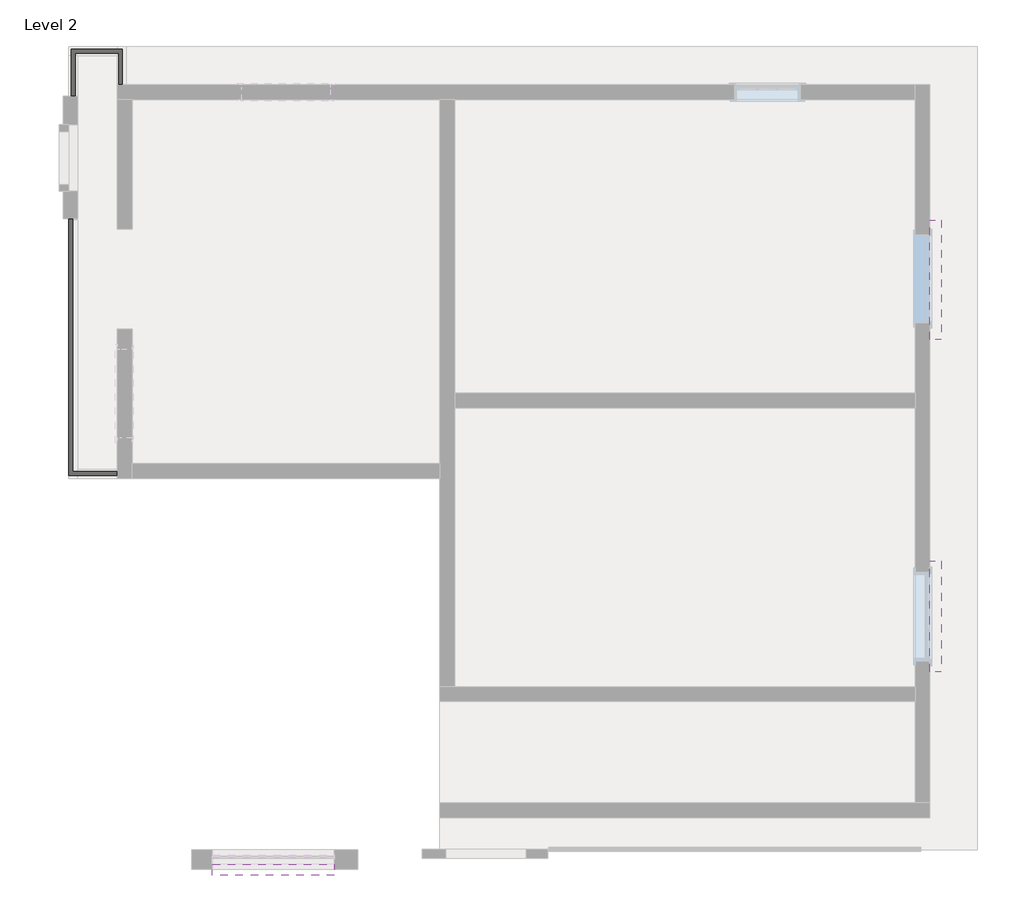
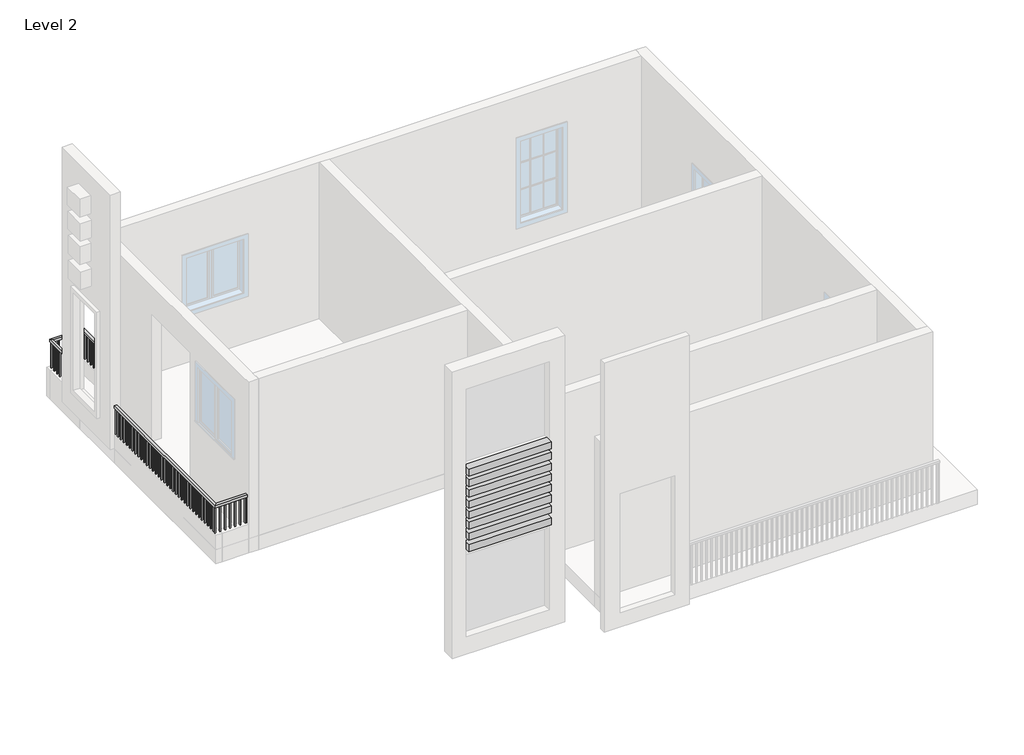
# One storey, part 2 of 2: 10 proxies, 2 railings.
"""IFC4 building model written with IfcOpenShell, lengths in millimetres."""

from ifc_helpers import new_model, si_unit, frame, origin, place, context, project, spatial, polyline, outline, extrude, faceted_brep, element, save

model = new_model("IFC4")

# Units and contexts
model_context = context("Model", 3, world=origin())
ifc_project = project(units=[si_unit("LENGTHUNIT", "METRE", prefix="MILLI")], contexts=[model_context])

# Site, building, storey
site = spatial("IfcSite", under=ifc_project)
building = spatial("IfcBuilding", under=site)
storey = spatial("IfcBuildingStorey", under=building, Name="Level 2", Elevation=3657.6)

# Proxies
placement = place(None, origin())
element("IfcBuildingElementProxy", 1, Name="Cornice", ObjectType="Cornice", at=placement, inside=storey, context=model_context, shape_type="SweptSolid", body=[
    extrude(outline(polyline([(-10477.4344883, -2980.8451776), (-10477.4344883, -2828.4451776), (-8801.0344883, -2828.4451776), (-8801.0344883, -2980.8451776), (-10477.4344883, -2980.8451776)])), frame((0.0, 0.0, 8153.4), z_axis=(0.0, 0.0, 1.0), x_axis=(1.0, 0.0, 0.0)), (0.0, 0.0, 1.0), 152.4),
])
element("IfcBuildingElementProxy", 2, Name="Cornice", ObjectType="Cornice", at=placement, inside=storey, context=model_context, shape_type="SweptSolid", body=[
    extrude(outline(polyline([(-10477.4344883, -2980.8451776), (-10477.4344883, -2828.4451776), (-8801.0344883, -2828.4451776), (-8801.0344883, -2980.8451776), (-10477.4344883, -2980.8451776)])), frame((0.0, 0.0, 7924.8), z_axis=(0.0, 0.0, 1.0), x_axis=(1.0, 0.0, 0.0)), (0.0, 0.0, 1.0), 152.4),
])
element("IfcBuildingElementProxy", 3, Name="Cornice", ObjectType="Cornice", at=placement, inside=storey, context=model_context, shape_type="SweptSolid", body=[
    extrude(outline(polyline([(-10477.4344883, -2980.8451776), (-10477.4344883, -2828.4451776), (-8801.0344883, -2828.4451776), (-8801.0344883, -2980.8451776), (-10477.4344883, -2980.8451776)])), frame((0.0, 0.0, 7696.2), z_axis=(0.0, 0.0, 1.0), x_axis=(1.0, 0.0, 0.0)), (0.0, 0.0, 1.0), 152.4),
])
element("IfcBuildingElementProxy", 4, Name="Cornice", ObjectType="Cornice", at=placement, inside=storey, context=model_context, shape_type="SweptSolid", body=[
    extrude(outline(polyline([(-10477.4344883, -2980.8451776), (-10477.4344883, -2828.4451776), (-8801.0344883, -2828.4451776), (-8801.0344883, -2980.8451776), (-10477.4344883, -2980.8451776)])), frame((0.0, 0.0, 7467.6), z_axis=(0.0, 0.0, 1.0), x_axis=(1.0, 0.0, 0.0)), (0.0, 0.0, 1.0), 152.4),
])
element("IfcBuildingElementProxy", 5, Name="Cornice", ObjectType="Cornice", at=placement, inside=storey, context=model_context, shape_type="SweptSolid", body=[
    extrude(outline(polyline([(-10477.4344883, -2980.8451776), (-10477.4344883, -2828.4451776), (-8801.0344883, -2828.4451776), (-8801.0344883, -2980.8451776), (-10477.4344883, -2980.8451776)])), frame((0.0, 0.0, 7239.0), z_axis=(0.0, 0.0, 1.0), x_axis=(1.0, 0.0, 0.0)), (0.0, 0.0, 1.0), 152.4),
])
element("IfcBuildingElementProxy", 6, Name="Cornice", ObjectType="Cornice", at=placement, inside=storey, context=model_context, shape_type="SweptSolid", body=[
    extrude(outline(polyline([(-10477.4344883, -2980.8451776), (-10477.4344883, -2828.4451776), (-8801.0344883, -2828.4451776), (-8801.0344883, -2980.8451776), (-10477.4344883, -2980.8451776)])), frame((0.0, 0.0, 7010.4), z_axis=(0.0, 0.0, 1.0), x_axis=(1.0, 0.0, 0.0)), (0.0, 0.0, 1.0), 152.4),
])
element("IfcBuildingElementProxy", 7, Name="Cornice", ObjectType="Cornice", at=placement, inside=storey, context=model_context, shape_type="SweptSolid", body=[
    extrude(outline(polyline([(-10477.4344883, -2980.8451776), (-10477.4344883, -2828.4451776), (-8801.0344883, -2828.4451776), (-8801.0344883, -2980.8451776), (-10477.4344883, -2980.8451776)])), frame((0.0, 0.0, 6781.8), z_axis=(0.0, 0.0, 1.0), x_axis=(1.0, 0.0, 0.0)), (0.0, 0.0, 1.0), 152.4),
])
element("IfcBuildingElementProxy", 8, Name="Cornice", ObjectType="Cornice", at=placement, inside=storey, context=model_context, shape_type="SweptSolid", body=[
    extrude(outline(polyline([(-10477.4344883, -2980.8451776), (-10477.4344883, -2828.4451776), (-8801.0344883, -2828.4451776), (-8801.0344883, -2980.8451776), (-10477.4344883, -2980.8451776)])), frame((0.0, 0.0, 6527.8), z_axis=(0.0, 0.0, 1.0), x_axis=(1.0, 0.0, 0.0)), (0.0, 0.0, 1.0), 152.4),
])
element("IfcBuildingElementProxy", 9, Name="Cornice", ObjectType="Cornice", at=placement, inside=storey, context=model_context, shape_type="SweptSolid", body=[
    extrude(outline(polyline([(-610.2932708, 1339.073901), (-457.8932708, 1339.073901), (-457.8932708, -184.926099), (-610.2932708, -184.926099), (-610.2932708, 1339.073901)])), frame((0.0, 0.0, 6096.0), z_axis=(0.0, 0.0, 1.0), x_axis=(1.0, 0.0, 0.0)), (0.0, 0.0, 1.0), 152.4),
])
element("IfcBuildingElementProxy", 10, Name="Cornice", ObjectType="Cornice", at=placement, inside=storey, context=model_context, shape_type="SweptSolid", body=[
    extrude(outline(polyline([(-610.2932708, 6032.9483652), (-457.8932708, 6032.9483652), (-457.8932708, 4387.073901), (-610.2932708, 4387.073901), (-610.2932708, 6032.9483652)])), frame((0.0, 0.0, 6096.0), z_axis=(0.0, 0.0, 1.0), x_axis=(1.0, 0.0, 0.0)), (0.0, 0.0, 1.0), 152.4),
])

# Railings
element("IfcRailing", 11, ObjectType="Handrail - Rectangular", at=placement, inside=storey, context=model_context, shape_type="SolidModel", body=[
    faceted_brep([(-11768.1083357, 7892.273901, 4876.8), (-11768.1083357, 7892.273901, 4826.0), (-11717.3083357, 7892.273901, 4826.0), (-11717.3083357, 7892.273901, 4876.8), (-11768.1083357, 8331.6483652, 4876.8), (-11768.1083357, 8331.6483652, 4826.0), (-11717.3083357, 8382.4483652, 4826.0), (-11717.3083357, 8382.4483652, 4876.8), (-12365.0083357, 8331.6483652, 4876.8), (-12365.0083357, 8331.6483652, 4826.0), (-12415.8083357, 8382.4483652, 4826.0), (-12415.8083357, 8382.4483652, 4876.8), (-12365.0083357, 7739.873901, 4876.8), (-12415.8083357, 7739.873901, 4876.8), (-12415.8083357, 7739.873901, 4826.0), (-12365.0083357, 7739.873901, 4826.0)], [[[0, 1, 2, 3]], [[1, 0, 4, 5]], [[2, 1, 5, 6]], [[3, 2, 6, 7]], [[0, 3, 7, 4]], [[5, 4, 8, 9]], [[6, 5, 9, 10]], [[7, 6, 10, 11]], [[4, 7, 11, 8]], [[12, 13, 14, 15]], [[9, 8, 12, 15]], [[10, 9, 15, 14]], [[11, 10, 14, 13]], [[8, 11, 13, 12]]]),
    extrude(outline(polyline([(-12399.9333357, 7756.9733652), (-12380.8833357, 7756.9733652), (-12380.8833357, 7737.9233652), (-12399.9333357, 7737.9233652), (-12399.9333357, 7756.9733652)])), frame((0.0, 0.0, 3962.4), z_axis=(0.0, 0.0, 1.0), x_axis=(1.0, 0.0, 0.0)), (0.0, 0.0, 1.0), 863.6),
    extrude(outline(polyline([(-12399.9333357, 7858.5733652), (-12380.8833357, 7858.5733652), (-12380.8833357, 7839.5233652), (-12399.9333357, 7839.5233652), (-12399.9333357, 7858.5733652)])), frame((0.0, 0.0, 3962.4), z_axis=(0.0, 0.0, 1.0), x_axis=(1.0, 0.0, 0.0)), (0.0, 0.0, 1.0), 863.6),
    extrude(outline(polyline([(-12399.9333357, 7960.1733652), (-12380.8833357, 7960.1733652), (-12380.8833357, 7941.1233652), (-12399.9333357, 7941.1233652), (-12399.9333357, 7960.1733652)])), frame((0.0, 0.0, 3962.4), z_axis=(0.0, 0.0, 1.0), x_axis=(1.0, 0.0, 0.0)), (0.0, 0.0, 1.0), 863.6),
    extrude(outline(polyline([(-12399.9333357, 8061.7733652), (-12380.8833357, 8061.7733652), (-12380.8833357, 8042.7233652), (-12399.9333357, 8042.7233652), (-12399.9333357, 8061.7733652)])), frame((0.0, 0.0, 3962.4), z_axis=(0.0, 0.0, 1.0), x_axis=(1.0, 0.0, 0.0)), (0.0, 0.0, 1.0), 863.6),
    extrude(outline(polyline([(-12399.9333357, 8163.3733652), (-12380.8833357, 8163.3733652), (-12380.8833357, 8144.3233652), (-12399.9333357, 8144.3233652), (-12399.9333357, 8163.3733652)])), frame((0.0, 0.0, 3962.4), z_axis=(0.0, 0.0, 1.0), x_axis=(1.0, 0.0, 0.0)), (0.0, 0.0, 1.0), 863.6),
    extrude(outline(polyline([(-12399.9333357, 8264.9733652), (-12380.8833357, 8264.9733652), (-12380.8833357, 8245.9233652), (-12399.9333357, 8245.9233652), (-12399.9333357, 8264.9733652)])), frame((0.0, 0.0, 3962.4), z_axis=(0.0, 0.0, 1.0), x_axis=(1.0, 0.0, 0.0)), (0.0, 0.0, 1.0), 863.6),
    extrude(outline(polyline([(-12342.7833357, 8366.5733652), (-12342.7833357, 8347.5233652), (-12361.8333357, 8347.5233652), (-12361.8333357, 8366.5733652), (-12342.7833357, 8366.5733652)])), frame((0.0, 0.0, 3962.4), z_axis=(0.0, 0.0, 1.0), x_axis=(1.0, 0.0, 0.0)), (0.0, 0.0, 1.0), 863.6),
    extrude(outline(polyline([(-12241.1833357, 8366.5733652), (-12241.1833357, 8347.5233652), (-12260.2333357, 8347.5233652), (-12260.2333357, 8366.5733652), (-12241.1833357, 8366.5733652)])), frame((0.0, 0.0, 3962.4), z_axis=(0.0, 0.0, 1.0), x_axis=(1.0, 0.0, 0.0)), (0.0, 0.0, 1.0), 863.6),
    extrude(outline(polyline([(-12139.5833357, 8366.5733652), (-12139.5833357, 8347.5233652), (-12158.6333357, 8347.5233652), (-12158.6333357, 8366.5733652), (-12139.5833357, 8366.5733652)])), frame((0.0, 0.0, 3962.4), z_axis=(0.0, 0.0, 1.0), x_axis=(1.0, 0.0, 0.0)), (0.0, 0.0, 1.0), 863.6),
    extrude(outline(polyline([(-12037.9833357, 8366.5733652), (-12037.9833357, 8347.5233652), (-12057.0333357, 8347.5233652), (-12057.0333357, 8366.5733652), (-12037.9833357, 8366.5733652)])), frame((0.0, 0.0, 3962.4), z_axis=(0.0, 0.0, 1.0), x_axis=(1.0, 0.0, 0.0)), (0.0, 0.0, 1.0), 863.6),
    extrude(outline(polyline([(-11936.3833357, 8366.5733652), (-11936.3833357, 8347.5233652), (-11955.4333357, 8347.5233652), (-11955.4333357, 8366.5733652), (-11936.3833357, 8366.5733652)])), frame((0.0, 0.0, 3962.4), z_axis=(0.0, 0.0, 1.0), x_axis=(1.0, 0.0, 0.0)), (0.0, 0.0, 1.0), 863.6),
    extrude(outline(polyline([(-11834.7833357, 8366.5733652), (-11834.7833357, 8347.5233652), (-11853.8333357, 8347.5233652), (-11853.8333357, 8366.5733652), (-11834.7833357, 8366.5733652)])), frame((0.0, 0.0, 3962.4), z_axis=(0.0, 0.0, 1.0), x_axis=(1.0, 0.0, 0.0)), (0.0, 0.0, 1.0), 863.6),
    extrude(outline(polyline([(-11733.1833357, 8289.148901), (-11752.2333357, 8289.148901), (-11752.2333357, 8308.198901), (-11733.1833357, 8308.198901), (-11733.1833357, 8289.148901)])), frame((0.0, 0.0, 3962.4), z_axis=(0.0, 0.0, 1.0), x_axis=(1.0, 0.0, 0.0)), (0.0, 0.0, 1.0), 863.6),
    extrude(outline(polyline([(-11733.1833357, 8187.548901), (-11752.2333357, 8187.548901), (-11752.2333357, 8206.598901), (-11733.1833357, 8206.598901), (-11733.1833357, 8187.548901)])), frame((0.0, 0.0, 3962.4), z_axis=(0.0, 0.0, 1.0), x_axis=(1.0, 0.0, 0.0)), (0.0, 0.0, 1.0), 863.6),
    extrude(outline(polyline([(-11733.1833357, 8085.948901), (-11752.2333357, 8085.948901), (-11752.2333357, 8104.998901), (-11733.1833357, 8104.998901), (-11733.1833357, 8085.948901)])), frame((0.0, 0.0, 3962.4), z_axis=(0.0, 0.0, 1.0), x_axis=(1.0, 0.0, 0.0)), (0.0, 0.0, 1.0), 863.6),
    extrude(outline(polyline([(-11733.1833357, 7984.348901), (-11752.2333357, 7984.348901), (-11752.2333357, 8003.398901), (-11733.1833357, 8003.398901), (-11733.1833357, 7984.348901)])), frame((0.0, 0.0, 3962.4), z_axis=(0.0, 0.0, 1.0), x_axis=(1.0, 0.0, 0.0)), (0.0, 0.0, 1.0), 863.6),
    extrude(outline(polyline([(-12380.8833357, 8366.5733652), (-12380.8833357, 8347.5233652), (-12399.9333357, 8347.5233652), (-12399.9333357, 8366.5733652), (-12380.8833357, 8366.5733652)])), frame((0.0, 0.0, 3962.4), z_axis=(0.0, 0.0, 1.0), x_axis=(1.0, 0.0, 0.0)), (0.0, 0.0, 1.0), 863.6),
    extrude(outline(polyline([(-11733.1833357, 8347.5233652), (-11752.2333357, 8347.5233652), (-11752.2333357, 8366.5733652), (-11733.1833357, 8366.5733652), (-11733.1833357, 8347.5233652)])), frame((0.0, 0.0, 3962.4), z_axis=(0.0, 0.0, 1.0), x_axis=(1.0, 0.0, 0.0)), (0.0, 0.0, 1.0), 863.6),
    extrude(outline(polyline([(-12399.9333357, 7758.923901), (-12380.8833357, 7758.923901), (-12380.8833357, 7739.873901), (-12399.9333357, 7739.873901), (-12399.9333357, 7758.923901)])), frame((0.0, 0.0, 3962.4), z_axis=(0.0, 0.0, 1.0), x_axis=(1.0, 0.0, 0.0)), (0.0, 0.0, 1.0), 863.6),
    extrude(outline(polyline([(-11733.1833357, 7892.273901), (-11752.2333357, 7892.273901), (-11752.2333357, 7911.323901), (-11733.1833357, 7911.323901), (-11733.1833357, 7892.273901)])), frame((0.0, 0.0, 3962.4), z_axis=(0.0, 0.0, 1.0), x_axis=(1.0, 0.0, 0.0)), (0.0, 0.0, 1.0), 863.6),
])
element("IfcRailing", 12, ObjectType="Handrail - Rectangular", at=placement, inside=storey, context=model_context, shape_type="SolidModel", body=[
    faceted_brep([(-12401.5677951, 6050.8287391, 4876.8), (-12401.5677951, 6050.8287391, 4826.0), (-12452.3677951, 6050.8287391, 4826.0), (-12452.3677951, 6050.8287391, 4876.8), (-12401.5677951, 2571.0287391, 4876.8), (-12401.5677951, 2571.0287391, 4826.0), (-12452.3677951, 2520.2287391, 4826.0), (-12452.3677951, 2520.2287391, 4876.8), (-11791.9677951, 2571.0287391, 4876.8), (-11791.9677951, 2520.2287391, 4876.8), (-11791.9677951, 2520.2287391, 4826.0), (-11791.9677951, 2571.0287391, 4826.0)], [[[0, 1, 2, 3]], [[1, 0, 4, 5]], [[2, 1, 5, 6]], [[3, 2, 6, 7]], [[0, 3, 7, 4]], [[8, 9, 10, 11]], [[5, 4, 8, 11]], [[6, 5, 11, 10]], [[7, 6, 10, 9]], [[4, 7, 9, 8]]]),
    extrude(outline(polyline([(-11826.8927951, 2536.1037391), (-11826.8927951, 2555.1537391), (-11807.8427951, 2555.1537391), (-11807.8427951, 2536.1037391), (-11826.8927951, 2536.1037391)])), frame((0.0, 0.0, 3962.4), z_axis=(0.0, 0.0, 1.0), x_axis=(1.0, 0.0, 0.0)), (0.0, 0.0, 1.0), 863.6),
    extrude(outline(polyline([(-11928.4927951, 2536.1037391), (-11928.4927951, 2555.1537391), (-11909.4427951, 2555.1537391), (-11909.4427951, 2536.1037391), (-11928.4927951, 2536.1037391)])), frame((0.0, 0.0, 3962.4), z_axis=(0.0, 0.0, 1.0), x_axis=(1.0, 0.0, 0.0)), (0.0, 0.0, 1.0), 863.6),
    extrude(outline(polyline([(-12030.0927951, 2536.1037391), (-12030.0927951, 2555.1537391), (-12011.0427951, 2555.1537391), (-12011.0427951, 2536.1037391), (-12030.0927951, 2536.1037391)])), frame((0.0, 0.0, 3962.4), z_axis=(0.0, 0.0, 1.0), x_axis=(1.0, 0.0, 0.0)), (0.0, 0.0, 1.0), 863.6),
    extrude(outline(polyline([(-12131.6927951, 2536.1037391), (-12131.6927951, 2555.1537391), (-12112.6427951, 2555.1537391), (-12112.6427951, 2536.1037391), (-12131.6927951, 2536.1037391)])), frame((0.0, 0.0, 3962.4), z_axis=(0.0, 0.0, 1.0), x_axis=(1.0, 0.0, 0.0)), (0.0, 0.0, 1.0), 863.6),
    extrude(outline(polyline([(-12233.2927951, 2536.1037391), (-12233.2927951, 2555.1537391), (-12214.2427951, 2555.1537391), (-12214.2427951, 2536.1037391), (-12233.2927951, 2536.1037391)])), frame((0.0, 0.0, 3962.4), z_axis=(0.0, 0.0, 1.0), x_axis=(1.0, 0.0, 0.0)), (0.0, 0.0, 1.0), 863.6),
    extrude(outline(polyline([(-12334.8927951, 2536.1037391), (-12334.8927951, 2555.1537391), (-12315.8427951, 2555.1537391), (-12315.8427951, 2536.1037391), (-12334.8927951, 2536.1037391)])), frame((0.0, 0.0, 3962.4), z_axis=(0.0, 0.0, 1.0), x_axis=(1.0, 0.0, 0.0)), (0.0, 0.0, 1.0), 863.6),
    extrude(outline(polyline([(-12436.4927951, 2605.9537391), (-12417.4427951, 2605.9537391), (-12417.4427951, 2586.9037391), (-12436.4927951, 2586.9037391), (-12436.4927951, 2605.9537391)])), frame((0.0, 0.0, 3962.4), z_axis=(0.0, 0.0, 1.0), x_axis=(1.0, 0.0, 0.0)), (0.0, 0.0, 1.0), 863.6),
    extrude(outline(polyline([(-12436.4927951, 2707.5537391), (-12417.4427951, 2707.5537391), (-12417.4427951, 2688.5037391), (-12436.4927951, 2688.5037391), (-12436.4927951, 2707.5537391)])), frame((0.0, 0.0, 3962.4), z_axis=(0.0, 0.0, 1.0), x_axis=(1.0, 0.0, 0.0)), (0.0, 0.0, 1.0), 863.6),
    extrude(outline(polyline([(-12436.4927951, 2809.1537391), (-12417.4427951, 2809.1537391), (-12417.4427951, 2790.1037391), (-12436.4927951, 2790.1037391), (-12436.4927951, 2809.1537391)])), frame((0.0, 0.0, 3962.4), z_axis=(0.0, 0.0, 1.0), x_axis=(1.0, 0.0, 0.0)), (0.0, 0.0, 1.0), 863.6),
    extrude(outline(polyline([(-12436.4927951, 2910.7537391), (-12417.4427951, 2910.7537391), (-12417.4427951, 2891.7037391), (-12436.4927951, 2891.7037391), (-12436.4927951, 2910.7537391)])), frame((0.0, 0.0, 3962.4), z_axis=(0.0, 0.0, 1.0), x_axis=(1.0, 0.0, 0.0)), (0.0, 0.0, 1.0), 863.6),
    extrude(outline(polyline([(-12436.4927951, 3012.3537391), (-12417.4427951, 3012.3537391), (-12417.4427951, 2993.3037391), (-12436.4927951, 2993.3037391), (-12436.4927951, 3012.3537391)])), frame((0.0, 0.0, 3962.4), z_axis=(0.0, 0.0, 1.0), x_axis=(1.0, 0.0, 0.0)), (0.0, 0.0, 1.0), 863.6),
    extrude(outline(polyline([(-12436.4927951, 3113.9537391), (-12417.4427951, 3113.9537391), (-12417.4427951, 3094.9037391), (-12436.4927951, 3094.9037391), (-12436.4927951, 3113.9537391)])), frame((0.0, 0.0, 3962.4), z_axis=(0.0, 0.0, 1.0), x_axis=(1.0, 0.0, 0.0)), (0.0, 0.0, 1.0), 863.6),
    extrude(outline(polyline([(-12436.4927951, 3215.5537391), (-12417.4427951, 3215.5537391), (-12417.4427951, 3196.5037391), (-12436.4927951, 3196.5037391), (-12436.4927951, 3215.5537391)])), frame((0.0, 0.0, 3962.4), z_axis=(0.0, 0.0, 1.0), x_axis=(1.0, 0.0, 0.0)), (0.0, 0.0, 1.0), 863.6),
    extrude(outline(polyline([(-12436.4927951, 3317.1537391), (-12417.4427951, 3317.1537391), (-12417.4427951, 3298.1037391), (-12436.4927951, 3298.1037391), (-12436.4927951, 3317.1537391)])), frame((0.0, 0.0, 3962.4), z_axis=(0.0, 0.0, 1.0), x_axis=(1.0, 0.0, 0.0)), (0.0, 0.0, 1.0), 863.6),
    extrude(outline(polyline([(-12436.4927951, 3418.7537391), (-12417.4427951, 3418.7537391), (-12417.4427951, 3399.7037391), (-12436.4927951, 3399.7037391), (-12436.4927951, 3418.7537391)])), frame((0.0, 0.0, 3962.4), z_axis=(0.0, 0.0, 1.0), x_axis=(1.0, 0.0, 0.0)), (0.0, 0.0, 1.0), 863.6),
    extrude(outline(polyline([(-12436.4927951, 3520.3537391), (-12417.4427951, 3520.3537391), (-12417.4427951, 3501.3037391), (-12436.4927951, 3501.3037391), (-12436.4927951, 3520.3537391)])), frame((0.0, 0.0, 3962.4), z_axis=(0.0, 0.0, 1.0), x_axis=(1.0, 0.0, 0.0)), (0.0, 0.0, 1.0), 863.6),
    extrude(outline(polyline([(-12436.4927951, 3621.9537391), (-12417.4427951, 3621.9537391), (-12417.4427951, 3602.9037391), (-12436.4927951, 3602.9037391), (-12436.4927951, 3621.9537391)])), frame((0.0, 0.0, 3962.4), z_axis=(0.0, 0.0, 1.0), x_axis=(1.0, 0.0, 0.0)), (0.0, 0.0, 1.0), 863.6),
    extrude(outline(polyline([(-12436.4927951, 3723.5537391), (-12417.4427951, 3723.5537391), (-12417.4427951, 3704.5037391), (-12436.4927951, 3704.5037391), (-12436.4927951, 3723.5537391)])), frame((0.0, 0.0, 3962.4), z_axis=(0.0, 0.0, 1.0), x_axis=(1.0, 0.0, 0.0)), (0.0, 0.0, 1.0), 863.6),
    extrude(outline(polyline([(-12436.4927951, 3825.1537391), (-12417.4427951, 3825.1537391), (-12417.4427951, 3806.1037391), (-12436.4927951, 3806.1037391), (-12436.4927951, 3825.1537391)])), frame((0.0, 0.0, 3962.4), z_axis=(0.0, 0.0, 1.0), x_axis=(1.0, 0.0, 0.0)), (0.0, 0.0, 1.0), 863.6),
    extrude(outline(polyline([(-12436.4927951, 3926.7537391), (-12417.4427951, 3926.7537391), (-12417.4427951, 3907.7037391), (-12436.4927951, 3907.7037391), (-12436.4927951, 3926.7537391)])), frame((0.0, 0.0, 3962.4), z_axis=(0.0, 0.0, 1.0), x_axis=(1.0, 0.0, 0.0)), (0.0, 0.0, 1.0), 863.6),
    extrude(outline(polyline([(-12436.4927951, 4028.3537391), (-12417.4427951, 4028.3537391), (-12417.4427951, 4009.3037391), (-12436.4927951, 4009.3037391), (-12436.4927951, 4028.3537391)])), frame((0.0, 0.0, 3962.4), z_axis=(0.0, 0.0, 1.0), x_axis=(1.0, 0.0, 0.0)), (0.0, 0.0, 1.0), 863.6),
    extrude(outline(polyline([(-12436.4927951, 4129.9537391), (-12417.4427951, 4129.9537391), (-12417.4427951, 4110.9037391), (-12436.4927951, 4110.9037391), (-12436.4927951, 4129.9537391)])), frame((0.0, 0.0, 3962.4), z_axis=(0.0, 0.0, 1.0), x_axis=(1.0, 0.0, 0.0)), (0.0, 0.0, 1.0), 863.6),
    extrude(outline(polyline([(-12436.4927951, 4231.5537391), (-12417.4427951, 4231.5537391), (-12417.4427951, 4212.5037391), (-12436.4927951, 4212.5037391), (-12436.4927951, 4231.5537391)])), frame((0.0, 0.0, 3962.4), z_axis=(0.0, 0.0, 1.0), x_axis=(1.0, 0.0, 0.0)), (0.0, 0.0, 1.0), 863.6),
    extrude(outline(polyline([(-12436.4927951, 4333.1537391), (-12417.4427951, 4333.1537391), (-12417.4427951, 4314.1037391), (-12436.4927951, 4314.1037391), (-12436.4927951, 4333.1537391)])), frame((0.0, 0.0, 3962.4), z_axis=(0.0, 0.0, 1.0), x_axis=(1.0, 0.0, 0.0)), (0.0, 0.0, 1.0), 863.6),
    extrude(outline(polyline([(-12436.4927951, 4434.7537391), (-12417.4427951, 4434.7537391), (-12417.4427951, 4415.7037391), (-12436.4927951, 4415.7037391), (-12436.4927951, 4434.7537391)])), frame((0.0, 0.0, 3962.4), z_axis=(0.0, 0.0, 1.0), x_axis=(1.0, 0.0, 0.0)), (0.0, 0.0, 1.0), 863.6),
    extrude(outline(polyline([(-12436.4927951, 4536.3537391), (-12417.4427951, 4536.3537391), (-12417.4427951, 4517.3037391), (-12436.4927951, 4517.3037391), (-12436.4927951, 4536.3537391)])), frame((0.0, 0.0, 3962.4), z_axis=(0.0, 0.0, 1.0), x_axis=(1.0, 0.0, 0.0)), (0.0, 0.0, 1.0), 863.6),
    extrude(outline(polyline([(-12436.4927951, 4637.9537391), (-12417.4427951, 4637.9537391), (-12417.4427951, 4618.9037391), (-12436.4927951, 4618.9037391), (-12436.4927951, 4637.9537391)])), frame((0.0, 0.0, 3962.4), z_axis=(0.0, 0.0, 1.0), x_axis=(1.0, 0.0, 0.0)), (0.0, 0.0, 1.0), 863.6),
    extrude(outline(polyline([(-12436.4927951, 4739.5537391), (-12417.4427951, 4739.5537391), (-12417.4427951, 4720.5037391), (-12436.4927951, 4720.5037391), (-12436.4927951, 4739.5537391)])), frame((0.0, 0.0, 3962.4), z_axis=(0.0, 0.0, 1.0), x_axis=(1.0, 0.0, 0.0)), (0.0, 0.0, 1.0), 863.6),
    extrude(outline(polyline([(-12436.4927951, 4841.1537391), (-12417.4427951, 4841.1537391), (-12417.4427951, 4822.1037391), (-12436.4927951, 4822.1037391), (-12436.4927951, 4841.1537391)])), frame((0.0, 0.0, 3962.4), z_axis=(0.0, 0.0, 1.0), x_axis=(1.0, 0.0, 0.0)), (0.0, 0.0, 1.0), 863.6),
    extrude(outline(polyline([(-12436.4927951, 4942.7537391), (-12417.4427951, 4942.7537391), (-12417.4427951, 4923.7037391), (-12436.4927951, 4923.7037391), (-12436.4927951, 4942.7537391)])), frame((0.0, 0.0, 3962.4), z_axis=(0.0, 0.0, 1.0), x_axis=(1.0, 0.0, 0.0)), (0.0, 0.0, 1.0), 863.6),
    extrude(outline(polyline([(-12436.4927951, 5044.3537391), (-12417.4427951, 5044.3537391), (-12417.4427951, 5025.3037391), (-12436.4927951, 5025.3037391), (-12436.4927951, 5044.3537391)])), frame((0.0, 0.0, 3962.4), z_axis=(0.0, 0.0, 1.0), x_axis=(1.0, 0.0, 0.0)), (0.0, 0.0, 1.0), 863.6),
    extrude(outline(polyline([(-12436.4927951, 5145.9537391), (-12417.4427951, 5145.9537391), (-12417.4427951, 5126.9037391), (-12436.4927951, 5126.9037391), (-12436.4927951, 5145.9537391)])), frame((0.0, 0.0, 3962.4), z_axis=(0.0, 0.0, 1.0), x_axis=(1.0, 0.0, 0.0)), (0.0, 0.0, 1.0), 863.6),
    extrude(outline(polyline([(-12436.4927951, 5247.5537391), (-12417.4427951, 5247.5537391), (-12417.4427951, 5228.5037391), (-12436.4927951, 5228.5037391), (-12436.4927951, 5247.5537391)])), frame((0.0, 0.0, 3962.4), z_axis=(0.0, 0.0, 1.0), x_axis=(1.0, 0.0, 0.0)), (0.0, 0.0, 1.0), 863.6),
    extrude(outline(polyline([(-12436.4927951, 5349.1537391), (-12417.4427951, 5349.1537391), (-12417.4427951, 5330.1037391), (-12436.4927951, 5330.1037391), (-12436.4927951, 5349.1537391)])), frame((0.0, 0.0, 3962.4), z_axis=(0.0, 0.0, 1.0), x_axis=(1.0, 0.0, 0.0)), (0.0, 0.0, 1.0), 863.6),
    extrude(outline(polyline([(-12436.4927951, 5450.7537391), (-12417.4427951, 5450.7537391), (-12417.4427951, 5431.7037391), (-12436.4927951, 5431.7037391), (-12436.4927951, 5450.7537391)])), frame((0.0, 0.0, 3962.4), z_axis=(0.0, 0.0, 1.0), x_axis=(1.0, 0.0, 0.0)), (0.0, 0.0, 1.0), 863.6),
    extrude(outline(polyline([(-12436.4927951, 5552.3537391), (-12417.4427951, 5552.3537391), (-12417.4427951, 5533.3037391), (-12436.4927951, 5533.3037391), (-12436.4927951, 5552.3537391)])), frame((0.0, 0.0, 3962.4), z_axis=(0.0, 0.0, 1.0), x_axis=(1.0, 0.0, 0.0)), (0.0, 0.0, 1.0), 863.6),
    extrude(outline(polyline([(-12436.4927951, 5653.9537391), (-12417.4427951, 5653.9537391), (-12417.4427951, 5634.9037391), (-12436.4927951, 5634.9037391), (-12436.4927951, 5653.9537391)])), frame((0.0, 0.0, 3962.4), z_axis=(0.0, 0.0, 1.0), x_axis=(1.0, 0.0, 0.0)), (0.0, 0.0, 1.0), 863.6),
    extrude(outline(polyline([(-12436.4927951, 5755.5537391), (-12417.4427951, 5755.5537391), (-12417.4427951, 5736.5037391), (-12436.4927951, 5736.5037391), (-12436.4927951, 5755.5537391)])), frame((0.0, 0.0, 3962.4), z_axis=(0.0, 0.0, 1.0), x_axis=(1.0, 0.0, 0.0)), (0.0, 0.0, 1.0), 863.6),
    extrude(outline(polyline([(-12436.4927951, 5857.1537391), (-12417.4427951, 5857.1537391), (-12417.4427951, 5838.1037391), (-12436.4927951, 5838.1037391), (-12436.4927951, 5857.1537391)])), frame((0.0, 0.0, 3962.4), z_axis=(0.0, 0.0, 1.0), x_axis=(1.0, 0.0, 0.0)), (0.0, 0.0, 1.0), 863.6),
    extrude(outline(polyline([(-12436.4927951, 5958.7537391), (-12417.4427951, 5958.7537391), (-12417.4427951, 5939.7037391), (-12436.4927951, 5939.7037391), (-12436.4927951, 5958.7537391)])), frame((0.0, 0.0, 3962.4), z_axis=(0.0, 0.0, 1.0), x_axis=(1.0, 0.0, 0.0)), (0.0, 0.0, 1.0), 863.6),
    extrude(outline(polyline([(-12436.4927951, 2555.1537391), (-12417.4427951, 2555.1537391), (-12417.4427951, 2536.1037391), (-12436.4927951, 2536.1037391), (-12436.4927951, 2555.1537391)])), frame((0.0, 0.0, 3962.4), z_axis=(0.0, 0.0, 1.0), x_axis=(1.0, 0.0, 0.0)), (0.0, 0.0, 1.0), 863.6),
    extrude(outline(polyline([(-11811.0177951, 2536.1037391), (-11811.0177951, 2555.1537391), (-11791.9677951, 2555.1537391), (-11791.9677951, 2536.1037391), (-11811.0177951, 2536.1037391)])), frame((0.0, 0.0, 3962.4), z_axis=(0.0, 0.0, 1.0), x_axis=(1.0, 0.0, 0.0)), (0.0, 0.0, 1.0), 863.6),
    extrude(outline(polyline([(-12436.4927951, 6050.8287391), (-12417.4427951, 6050.8287391), (-12417.4427951, 6031.7787391), (-12436.4927951, 6031.7787391), (-12436.4927951, 6050.8287391)])), frame((0.0, 0.0, 3962.4), z_axis=(0.0, 0.0, 1.0), x_axis=(1.0, 0.0, 0.0)), (0.0, 0.0, 1.0), 863.6),
])

save(model, "model.ifc")

# Revit data of these elements
# Type "Handrail - Rectangular"
#   Assembly Code = "C2010400"
#   built-in parameter 1008612 = 0.0416667 (stored number, unit not read)
#   built-in parameter 1008611 = 0.0416667 (stored number, unit not read)
#   built-in parameter 1008609 = 0.333333 (stored number, unit not read)
#   built-in parameter 1008604 = 0.166667 (stored number, unit not read)
#   built-in parameter 1008603 = 0.166667 (stored number, unit not read)
#   Railing Height = 3' - 0"
#   built-in parameter 1008630 = 2
#   built-in parameter 1008610 = 2
#   built-in parameter 1008618 = Baluster - Square : 3/4"
# Elements 1, 2, 3, 4, 5, 6, 7, 8, 9, 10 (IfcBuildingElementProxy, "Cornice")
#   Phase Created = New Construction
#   Materials on its faces: "Default Wall"
# Elements 11, 12 (IfcRailing, "Handrail - Rectangular")
#   built-in parameter 1008621 = 1 (stored number, unit not read)
#   Phase Created = New Construction
# Materials
#   "Default Wall": colour RGB 128 128 128, transparency 0
